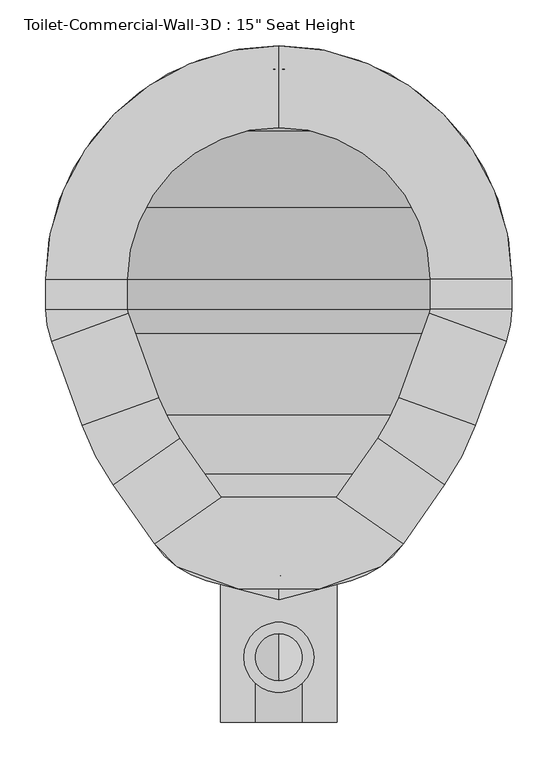
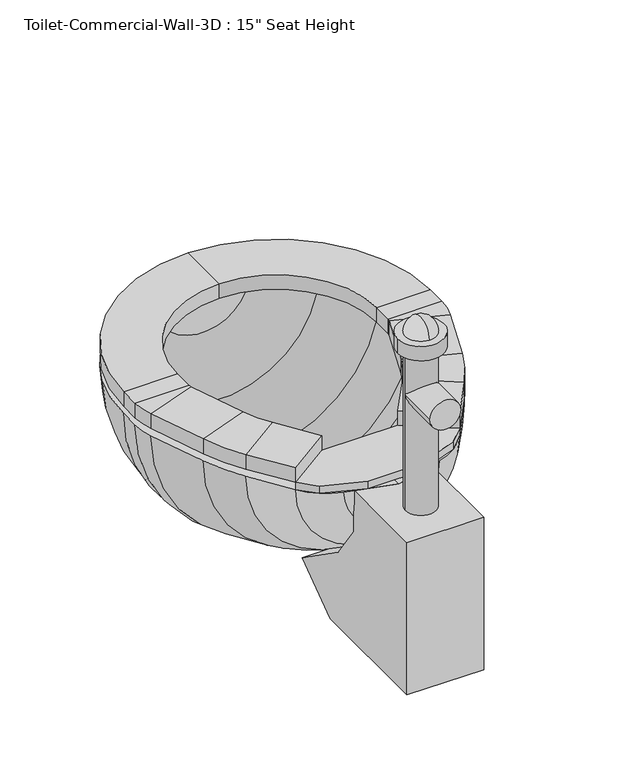
"""IFC4 building model written with IfcOpenShell, lengths in millimetres: flow terminal geometry."""

from ifc_helpers import new_model, si_unit, point, frame, frame_2d, origin, place, context, project, spatial, polyline, circle_curve, ellipse_curve, trimmed, segment, composite_curve, outline, extrude, source, transform, mapped, element, save
from ifc_brep_helpers import plane_surface, cylinder_surface, revolved_surface, advanced_brep


def flow_terminal_6d55091a(model_context):
    return source(origin(), model_context, "Body", "SolidModel", [
        extrude(outline(polyline([(467.7541169, 321.2347495), (540.5767337, 270.2438043), (515.6262519, 245.2933226), (449.563909, 221.2485961), (360.2423986, 221.2485961), (294.1800557, 245.2933226), (269.229574, 270.2438043), (342.0521907, 321.2347495), (467.7541169, 321.2347495)])), frame((0.0, 0.0, 342.9), z_axis=(0.0, 0.0, 1.0), x_axis=(1.0, 0.0, 0.0)), (0.0, 0.0, 1.0), 12.7),
        advanced_brep(
        [(467.7541169, 321.2347495, 355.6), (540.5767337, 270.2438043, 355.6), (540.5767337, 270.2438043, 381.0), (467.7541169, 321.2347495, 381.0), (512.8583992, 385.6503403, 355.6), (585.6810159, 334.6593951, 355.6), (585.6810159, 334.6593951, 381.0), (512.8583992, 385.6503403, 381.0), (619.360053, 399.3562234, 355.6), (535.821379, 429.7618141, 355.6), (619.360053, 399.3562234, 381.0), (535.821379, 429.7618141, 381.0), (569.2372501, 521.5711654, 355.6), (652.7759241, 491.1655747, 355.6), (652.7759241, 491.1655747, 381.0), (569.2372501, 521.5711654, 381.0), (658.9031538, 525.9148212, 355.6), (570.0031538, 525.9148212, 355.6), (658.9031538, 525.9148212, 381.0), (570.0031538, 525.9148212, 381.0), (570.0031538, 558.8, 355.6), (658.9031538, 558.8, 355.6), (658.9031538, 558.8, 381.0), (570.0031538, 558.8, 381.0), (404.9031538, 812.8, 355.6), (404.9031538, 723.9, 355.6), (404.9031538, 812.8, 381.0), (404.9031538, 723.9, 381.0), (150.9031538, 558.8, 355.6), (239.8031538, 558.8, 355.6), (150.9031538, 558.8, 381.0), (239.8031538, 558.8, 381.0), (239.8031538, 525.9148212, 355.6), (150.9031538, 525.9148212, 355.6), (150.9031538, 525.9148212, 381.0), (239.8031538, 525.9148212, 381.0), (157.0303835, 491.1655747, 355.6), (240.5690575, 521.5711654, 355.6), (157.0303835, 491.1655747, 381.0), (240.5690575, 521.5711654, 381.0), (273.9849286, 429.7618141, 355.6), (190.4462546, 399.3562234, 355.6), (190.4462546, 399.3562234, 381.0), (273.9849286, 429.7618141, 381.0), (224.1252917, 334.6593951, 355.6), (296.9479084, 385.6503403, 355.6), (224.1252917, 334.6593951, 381.0), (296.9479084, 385.6503403, 381.0), (342.0521907, 321.2347495, 355.6), (342.0521907, 321.2347495, 381.0), (269.229574, 270.2438043, 381.0), (269.229574, 270.2438043, 355.6)],
        [
            (0, 1),
            (1, 2),
            (2, 3),
            (3, 0),
            (0, 4),
            (4, 5),
            (5, 1),
            (5, 6),
            (6, 2),
            (6, 7),
            (7, 3),
            (7, 4),
            (8, 5, circle_curve(frame((356.8099347, 494.9166514, 355.6), z_axis=(0.0, 0.0, -1.0), x_axis=(0.81915204428899, -0.5735764363510486, 0.0)), 279.4)),
            (4, 9, circle_curve(frame((356.8099347, 494.9166514, 355.6), z_axis=(0.0, 0.0, 1.0), x_axis=(0.81915204428899, -0.5735764363510486, 0.0)), 190.5)),
            (9, 8),
            (10, 6, circle_curve(frame((356.8099347, 494.9166514, 381.0), z_axis=(0.0, 0.0, -1.0), x_axis=(0.81915204428899, -0.5735764363510486, 0.0)), 279.4)),
            (8, 10),
            (11, 7, circle_curve(frame((356.8099347, 494.9166514, 381.0), z_axis=(0.0, 0.0, -1.0), x_axis=(0.81915204428899, -0.5735764363510486, 0.0)), 190.5)),
            (10, 11),
            (11, 9),
            (9, 12),
            (12, 13),
            (13, 8),
            (13, 14),
            (14, 10),
            (14, 15),
            (15, 11),
            (15, 12),
            (16, 13, circle_curve(frame((557.3031538, 525.9148212, 355.6), z_axis=(0.0, 0.0, -1.0), x_axis=(0.939692620785906, -0.34202014332567526, 0.0)), 101.6)),
            (12, 17, circle_curve(frame((557.3031538, 525.9148212, 355.6), z_axis=(0.0, 0.0, 1.0), x_axis=(0.939692620785906, -0.34202014332567526, 0.0)), 12.7)),
            (17, 16),
            (18, 14, circle_curve(frame((557.3031538, 525.9148212, 381.0), z_axis=(0.0, 0.0, -1.0), x_axis=(0.939692620785906, -0.34202014332567526, 0.0)), 101.6)),
            (16, 18),
            (19, 15, circle_curve(frame((557.3031538, 525.9148212, 381.0), z_axis=(0.0, 0.0, -1.0), x_axis=(0.939692620785906, -0.34202014332567526, 0.0)), 12.7)),
            (18, 19),
            (19, 17),
            (17, 20),
            (20, 21),
            (21, 16),
            (21, 22),
            (22, 18),
            (22, 23),
            (23, 19),
            (23, 20),
            (24, 21, circle_curve(frame((404.9031538, 558.8, 355.6), z_axis=(0.0, 0.0, -1.0), x_axis=(1.0, 0.0, 0.0)), 254.0)),
            (20, 25, circle_curve(frame((404.9031538, 558.8, 355.6), z_axis=(0.0, 0.0, 1.0), x_axis=(1.0, 0.0, 0.0)), 165.1)),
            (25, 24),
            (26, 22, circle_curve(frame((404.9031538, 558.8, 381.0), z_axis=(0.0, 0.0, -1.0), x_axis=(1.0, 0.0, 0.0)), 254.0)),
            (24, 26),
            (27, 23, circle_curve(frame((404.9031538, 558.8, 381.0), z_axis=(0.0, 0.0, -1.0), x_axis=(1.0, 0.0, 0.0)), 165.1)),
            (26, 27),
            (27, 25),
            (28, 24, circle_curve(frame((404.9031538, 558.8, 355.6), z_axis=(0.0, 0.0, -1.0), x_axis=(0.0, 1.0, 0.0)), 254.0)),
            (25, 29, circle_curve(frame((404.9031538, 558.8, 355.6), z_axis=(0.0, 0.0, 1.0), x_axis=(0.0, 1.0, 0.0)), 165.1)),
            (29, 28),
            (30, 26, circle_curve(frame((404.9031538, 558.8, 381.0), z_axis=(0.0, 0.0, -1.0), x_axis=(0.0, 1.0, 0.0)), 254.0)),
            (28, 30),
            (31, 27, circle_curve(frame((404.9031538, 558.8, 381.0), z_axis=(0.0, 0.0, -1.0), x_axis=(0.0, 1.0, 0.0)), 165.1)),
            (30, 31),
            (31, 29),
            (29, 32),
            (32, 33),
            (33, 28),
            (33, 34),
            (34, 30),
            (34, 35),
            (35, 31),
            (35, 32),
            (36, 33, circle_curve(frame((252.5031538, 525.9148212, 355.6), z_axis=(0.0, 0.0, -1.0), x_axis=(-1.0, 0.0, 0.0)), 101.6)),
            (32, 37, circle_curve(frame((252.5031538, 525.9148212, 355.6), z_axis=(0.0, 0.0, 1.0), x_axis=(-1.0, 0.0, 0.0)), 12.7)),
            (37, 36),
            (38, 34, circle_curve(frame((252.5031538, 525.9148212, 381.0), z_axis=(0.0, 0.0, -1.0), x_axis=(-1.0, 0.0, 0.0)), 101.6)),
            (36, 38),
            (39, 35, circle_curve(frame((252.5031538, 525.9148212, 381.0), z_axis=(0.0, 0.0, -1.0), x_axis=(-1.0, 0.0, 0.0)), 12.7)),
            (38, 39),
            (39, 37),
            (37, 40),
            (40, 41),
            (41, 36),
            (41, 42),
            (42, 38),
            (42, 43),
            (43, 39),
            (43, 40),
            (44, 41, circle_curve(frame((452.9963729, 494.9166514, 355.6), z_axis=(0.0, 0.0, -1.0), x_axis=(-0.9396926207859088, -0.34202014332566766, 0.0)), 279.4)),
            (40, 45, circle_curve(frame((452.9963729, 494.9166514, 355.6), z_axis=(0.0, 0.0, 1.0), x_axis=(-0.9396926207859088, -0.34202014332566766, 0.0)), 190.5)),
            (45, 44),
            (46, 42, circle_curve(frame((452.9963729, 494.9166514, 381.0), z_axis=(0.0, 0.0, -1.0), x_axis=(-0.9396926207859088, -0.34202014332566766, 0.0)), 279.4)),
            (44, 46),
            (47, 43, circle_curve(frame((452.9963729, 494.9166514, 381.0), z_axis=(0.0, 0.0, -1.0), x_axis=(-0.9396926207859088, -0.34202014332566766, 0.0)), 190.5)),
            (46, 47),
            (47, 45),
            (48, 49),
            (49, 50),
            (50, 51),
            (51, 48),
            (45, 48),
            (51, 44),
            (50, 46),
            (49, 47),
        ],
        [
            plane_surface(frame((540.5767337, 270.2438043, 439.6203184), z_axis=(-0.5735764363510434, -0.8191520442889938, 0.0), x_axis=(0.8191520442889938, -0.5735764363510434, 0.0))),
            plane_surface(frame((467.7541169, 321.2347495, 355.6), z_axis=(0.0, 0.0, -1.0), x_axis=(0.573576436351044, 0.8191520442889932, 0.0))),
            plane_surface(frame((540.5767337, 270.2438043, 355.6), z_axis=(0.8191520442889938, -0.5735764363510433, 0.0), x_axis=(0.5735764363510433, 0.8191520442889938, 0.0))),
            plane_surface(frame((540.5767337, 270.2438043, 381.0), z_axis=(0.0, 0.0, 1.0), x_axis=(0.5735764363510433, 0.8191520442889938, 0.0))),
            plane_surface(frame((467.7541169, 321.2347495, 381.0), z_axis=(-0.8191520442889932, 0.573576436351044, 0.0), x_axis=(0.573576436351044, 0.8191520442889932, 0.0))),
            plane_surface(frame((356.8099347, 494.9166514, 355.6), z_axis=(0.0, 0.0, -1.0), x_axis=(0.81915204428899, -0.5735764363510486, 0.0))),
            cylinder_surface(frame((356.8099347, 494.9166514, 342.9), z_axis=(0.0, 0.0, 1.0), x_axis=(0.81915204428899, -0.5735764363510486, 0.0)), 279.4),
            plane_surface(frame((356.8099347, 494.9166514, 381.0), z_axis=(0.0, 0.0, 1.0), x_axis=(0.81915204428899, -0.5735764363510486, 0.0))),
            revolved_surface(polyline([(512.8583991370526, 385.65034027512525, 381.0), (512.8583991370526, 385.65034027512525, 355.6)]), (356.8099347, 494.9166514, 342.9), (0.0, 0.0, 1.0)),
            plane_surface(frame((535.821379, 429.7618141, 355.6), z_axis=(0.0, 0.0, -1.0000000000000002), x_axis=(0.3420201433256694, 0.9396926207859082, 0.0))),
            plane_surface(frame((619.360053, 399.3562234, 355.6), z_axis=(0.9396926207859075, -0.34202014332567104, 0.0), x_axis=(0.34202014332567104, 0.9396926207859075, 0.0))),
            plane_surface(frame((619.360053, 399.3562234, 381.0), z_axis=(0.0, 0.0, 1.0), x_axis=(0.3420201433256696, 0.9396926207859081, 0.0))),
            plane_surface(frame((535.821379, 429.7618141, 381.0), z_axis=(-0.939692620785908, 0.34202014332567, 0.0), x_axis=(0.34202014332567, 0.939692620785908, 0.0))),
            plane_surface(frame((557.3031538, 525.9148212, 355.6), z_axis=(0.0, 0.0, -1.0), x_axis=(0.939692620785906, -0.34202014332567526, 0.0))),
            cylinder_surface(frame((557.3031538, 525.9148212, 342.9), z_axis=(0.0, 0.0, 1.0), x_axis=(0.939692620785906, -0.34202014332567526, 0.0)), 101.6),
            plane_surface(frame((557.3031538, 525.9148212, 381.0), z_axis=(0.0, 0.0, 1.0), x_axis=(0.939692620785906, -0.34202014332567526, 0.0))),
            revolved_surface(polyline([(569.237250083981, 521.5711653797639, 381.0), (569.237250083981, 521.5711653797639, 355.6)]), (557.3031538, 525.9148212, 342.9), (0.0, 0.0, 1.0)),
            plane_surface(frame((570.0031538, 525.9148212, 355.6), z_axis=(0.0, 0.0, -1.0), x_axis=(0.0, 1.0, 0.0))),
            plane_surface(frame((658.9031538, 525.9148212, 355.6), z_axis=(1.0, 0.0, 0.0), x_axis=(0.0, 1.0, 0.0))),
            plane_surface(frame((658.9031538, 525.9148212, 381.0), z_axis=(0.0, 0.0, 1.0), x_axis=(0.0, 1.0, 0.0))),
            plane_surface(frame((570.0031538, 525.9148212, 381.0), z_axis=(-1.0, 0.0, 0.0), x_axis=(0.0, 1.0, 0.0))),
            plane_surface(frame((404.9031538, 558.8, 355.6), z_axis=(0.0, 0.0, -1.0), x_axis=(1.0, 0.0, 0.0))),
            cylinder_surface(frame((404.9031538, 558.8, 342.9), z_axis=(0.0, 0.0, 1.0), x_axis=(1.0, 0.0, 0.0)), 254.0),
            plane_surface(frame((404.9031538, 558.8, 381.0), z_axis=(0.0, 0.0, 1.0), x_axis=(1.0, 0.0, 0.0))),
            revolved_surface(polyline([(570.0031538, 558.8, 381.0), (570.0031538, 558.8, 355.6)]), (404.9031538, 558.8, 342.9), (0.0, 0.0, 1.0)),
            plane_surface(frame((404.9031538, 558.8, 355.6), z_axis=(0.0, 0.0, -1.0), x_axis=(0.0, 1.0, 0.0))),
            cylinder_surface(frame((404.9031538, 558.8, 342.9), z_axis=(0.0, 0.0, 1.0), x_axis=(0.0, 1.0, 0.0)), 254.0),
            plane_surface(frame((404.9031538, 558.8, 381.0), z_axis=(0.0, 0.0, 1.0), x_axis=(0.0, 1.0, 0.0))),
            revolved_surface(polyline([(404.9031538, 723.9, 381.0), (404.9031538, 723.9, 355.6)]), (404.9031538, 558.8, 342.9), (0.0, 0.0, 1.0)),
            plane_surface(frame((239.8031538, 558.8, 355.6), z_axis=(0.0, 0.0, -1.0), x_axis=(0.0, -1.0, 0.0))),
            plane_surface(frame((150.9031538, 558.8, 355.6), z_axis=(-1.0, 0.0, 0.0), x_axis=(0.0, -1.0, 0.0))),
            plane_surface(frame((150.9031538, 558.8, 381.0), z_axis=(0.0, 0.0, 1.0), x_axis=(0.0, -1.0, 0.0))),
            plane_surface(frame((239.8031538, 558.8, 381.0), z_axis=(1.0, 0.0, 0.0), x_axis=(0.0, -1.0, 0.0))),
            plane_surface(frame((252.5031538, 525.9148212, 355.6), z_axis=(0.0, 0.0, -1.0), x_axis=(-1.0, 0.0, 0.0))),
            cylinder_surface(frame((252.5031538, 525.9148212, 342.9), z_axis=(0.0, 0.0, 1.0), x_axis=(-1.0, 0.0, 0.0)), 101.6),
            plane_surface(frame((252.5031538, 525.9148212, 381.0), z_axis=(0.0, 0.0, 1.0), x_axis=(-1.0, 0.0, 0.0))),
            revolved_surface(polyline([(239.80315380000002, 525.9148212, 381.0), (239.80315380000002, 525.9148212, 355.6)]), (252.5031538, 525.9148212, 342.9), (0.0, 0.0, 1.0)),
            plane_surface(frame((240.5690575, 521.5711654, 355.6), z_axis=(0.0, 0.0, -1.0), x_axis=(0.3420201433256672, -0.939692620785909, 0.0))),
            plane_surface(frame((157.0303835, 491.1655747, 355.6), z_axis=(-0.9396926207859091, -0.3420201433256668, 0.0), x_axis=(0.3420201433256668, -0.9396926207859091, 0.0))),
            plane_surface(frame((157.0303835, 491.1655747, 381.0), z_axis=(0.0, 0.0, 1.0), x_axis=(0.3420201433256671, -0.939692620785909, 0.0))),
            plane_surface(frame((240.5690575, 521.5711654, 381.0), z_axis=(0.9396926207859091, 0.342020143325667, 0.0), x_axis=(0.342020143325667, -0.9396926207859091, 0.0))),
            plane_surface(frame((452.9963729, 494.9166514, 355.6), z_axis=(0.0, 0.0, -1.0), x_axis=(-0.9396926207859088, -0.34202014332566766, 0.0))),
            cylinder_surface(frame((452.9963729, 494.9166514, 342.9), z_axis=(0.0, 0.0, 1.0), x_axis=(-0.9396926207859088, -0.34202014332566766, 0.0)), 279.4),
            plane_surface(frame((452.9963729, 494.9166514, 381.0), z_axis=(0.0, 0.0, 1.0), x_axis=(-0.9396926207859088, -0.34202014332566766, 0.0))),
            revolved_surface(polyline([(273.98492864028435, 429.7618140964603, 381.0), (273.98492864028435, 429.7618140964603, 355.6)]), (452.9963729, 494.9166514, 342.9), (0.0, 0.0, 1.0)),
            plane_surface(frame((269.229574, 270.2438043, 246.1796816), z_axis=(0.5735764363510462, -0.8191520442889919, 0.0), x_axis=(0.8191520442889919, 0.5735764363510462, 0.0))),
            plane_surface(frame((296.9479084, 385.6503403, 355.6), z_axis=(0.0, 0.0, -1.0), x_axis=(0.5735764363510465, -0.8191520442889916, 0.0))),
            plane_surface(frame((224.1252917, 334.6593951, 355.6), z_axis=(-0.8191520442889917, -0.5735764363510464, 0.0), x_axis=(0.5735764363510464, -0.8191520442889917, 0.0))),
            plane_surface(frame((224.1252917, 334.6593951, 381.0), z_axis=(0.0, 0.0, 1.0000000000000002), x_axis=(0.5735764363510462, -0.8191520442889919, 0.0))),
            plane_surface(frame((296.9479084, 385.6503403, 381.0), z_axis=(0.8191520442889916, 0.5735764363510465, 0.0), x_axis=(0.5735764363510465, -0.8191520442889916, 0.0))),
        ],
        [
            (0, [[1, 2, 3, 4]]),
            (1, [[-1, 5, 6, 7]]),
            (2, [[-2, -7, 8, 9]]),
            (3, [[-3, -9, 10, 11]]),
            (4, [[-4, -11, 12, -5]]),
            (5, [[13, -6, 14, 15]]),
            (6, [[16, -8, -13, 17]]),
            (7, [[18, -10, -16, 19]]),
            (8, [[-14, -12, -18, 20]]),
            (9, [[-15, 21, 22, 23]]),
            (10, [[-17, -23, 24, 25]]),
            (11, [[-19, -25, 26, 27]]),
            (12, [[-20, -27, 28, -21]]),
            (13, [[29, -22, 30, 31]]),
            (14, [[32, -24, -29, 33]]),
            (15, [[34, -26, -32, 35]]),
            (16, [[-30, -28, -34, 36]]),
            (17, [[-31, 37, 38, 39]]),
            (18, [[-33, -39, 40, 41]]),
            (19, [[-35, -41, 42, 43]]),
            (20, [[-36, -43, 44, -37]]),
            (21, [[45, -38, 46, 47]]),
            (22, [[48, -40, -45, 49]]),
            (23, [[50, -42, -48, 51]]),
            (24, [[-46, -44, -50, 52]]),
            (25, [[53, -47, 54, 55]]),
            (26, [[56, -49, -53, 57]]),
            (27, [[58, -51, -56, 59]]),
            (28, [[-54, -52, -58, 60]]),
            (29, [[-55, 61, 62, 63]]),
            (30, [[-57, -63, 64, 65]]),
            (31, [[-59, -65, 66, 67]]),
            (32, [[-60, -67, 68, -61]]),
            (33, [[69, -62, 70, 71]]),
            (34, [[72, -64, -69, 73]]),
            (35, [[74, -66, -72, 75]]),
            (36, [[-70, -68, -74, 76]]),
            (37, [[-71, 77, 78, 79]]),
            (38, [[-73, -79, 80, 81]]),
            (39, [[-75, -81, 82, 83]]),
            (40, [[-76, -83, 84, -77]]),
            (41, [[85, -78, 86, 87]]),
            (42, [[88, -80, -85, 89]]),
            (43, [[90, -82, -88, 91]]),
            (44, [[-86, -84, -90, 92]]),
            (45, [[93, 94, 95, 96]]),
            (46, [[-87, 97, -96, 98]]),
            (47, [[-89, -98, -95, 99]]),
            (48, [[-91, -99, -94, 100]]),
            (49, [[-92, -100, -93, -97]]),
        ],
    ),
        advanced_brep(
        [(491.7762702, 797.4819257, 342.9), (404.9031538, 812.8, 342.9), (404.9031538, 787.4, 342.9), (483.0889586, 773.6137331, 342.9), (566.547764, 720.4446102, 342.9), (619.7168869, 636.9858048, 342.9), (633.5031538, 558.8, 342.9), (633.5031538, 525.9148212, 342.9), (628.9077315, 499.8528863, 342.9), (596.6355667, 411.1858422, 342.9), (562.9565296, 346.4890139, 342.9), (525.0728964, 292.3855786, 342.9), (468.1430637, 252.5228806, 342.9), (404.9031538, 235.5777978, 342.9), (404.9031538, 209.2817829, 342.9), (483.6469009, 230.3811063, 342.9), (540.5767337, 270.2438043, 342.9), (585.6810159, 334.6593951, 342.9), (619.360053, 399.3562234, 342.9), (652.7759241, 491.1655747, 342.9), (658.9031538, 525.9148212, 342.9), (658.9031538, 558.8, 342.9), (643.5850795, 645.6731164, 342.9), (584.5082762, 738.4051224, 342.9), (318.0300374, 797.4819257, 342.9), (225.2980314, 738.4051224, 342.9), (166.2212281, 645.6731164, 342.9), (150.9031538, 558.8, 342.9), (150.9031538, 525.9148212, 342.9), (157.0303835, 491.1655747, 342.9), (190.4462546, 399.3562234, 342.9), (224.1252917, 334.6593951, 342.9), (269.229574, 270.2438043, 342.9), (326.1594067, 230.3811063, 342.9), (341.663244, 252.5228806, 342.9), (284.7334112, 292.3855786, 342.9), (246.849778, 346.4890139, 342.9), (213.1707409, 411.1858422, 342.9), (180.8985761, 499.8528863, 342.9), (176.3031538, 525.9148212, 342.9), (176.3031538, 558.8, 342.9), (190.0894207, 636.9858048, 342.9), (243.2585436, 720.4446102, 342.9), (326.7173491, 773.6137331, 342.9)],
        [
            (0, 1, circle_curve(frame((404.9031538, 558.8, 342.9), z_axis=(0.0, 0.0, 1.0), x_axis=(1.0, 0.0, 0.0)), 254.0)),
            (1, 2),
            (2, 3, circle_curve(frame((404.9031538, 558.8, 342.9), z_axis=(0.0, 0.0, -1.0), x_axis=(1.0, 0.0, 0.0)), 228.6)),
            (3, 4, circle_curve(frame((404.9031538, 558.8, 342.9), z_axis=(0.0, 0.0, -1.0), x_axis=(1.0, 0.0, 0.0)), 228.6)),
            (4, 5, circle_curve(frame((404.9031538, 558.8, 342.9), z_axis=(0.0, 0.0, -1.0), x_axis=(1.0, 0.0, 0.0)), 228.6)),
            (5, 6, circle_curve(frame((404.9031538, 558.8, 342.9), z_axis=(0.0, 0.0, -1.0), x_axis=(1.0, 0.0, 0.0)), 228.6)),
            (6, 7),
            (7, 8, circle_curve(frame((557.3031538, 525.9148212, 342.9), z_axis=(0.0, 0.0, -1.0), x_axis=(1.0, 0.0, 0.0)), 76.2)),
            (8, 9),
            (9, 10, circle_curve(frame((334.0854485, 506.7462703, 342.9), z_axis=(0.0, 0.0, -1.0), x_axis=(1.0, 0.0, 0.0)), 279.4)),
            (10, 11),
            (11, 12, circle_curve(frame((441.8470487, 350.6609446, 342.9), z_axis=(0.0, 0.0, -1.0), x_axis=(1.0, 0.0, 0.0)), 101.6)),
            (12, 13),
            (13, 14),
            (14, 15),
            (15, 16, circle_curve(frame((457.350886, 328.5191703, 342.9), z_axis=(0.0, 0.0, 1.0), x_axis=(1.0, 0.0, 0.0)), 101.6)),
            (16, 17),
            (17, 18, circle_curve(frame((356.8099347, 494.9166514, 342.9), z_axis=(0.0, 0.0, 1.0), x_axis=(1.0, 0.0, 0.0)), 279.4)),
            (18, 19),
            (19, 20, circle_curve(frame((557.3031538, 525.9148212, 342.9), z_axis=(0.0, 0.0, 1.0), x_axis=(1.0, 0.0, 0.0)), 101.6)),
            (20, 21),
            (21, 22, circle_curve(frame((404.9031538, 558.8, 342.9), z_axis=(0.0, 0.0, 1.0), x_axis=(1.0, 0.0, 0.0)), 254.0)),
            (22, 23, circle_curve(frame((404.9031538, 558.8, 342.9), z_axis=(0.0, 0.0, 1.0), x_axis=(1.0, 0.0, 0.0)), 254.0)),
            (23, 0, circle_curve(frame((404.9031538, 558.8, 342.9), z_axis=(0.0, 0.0, 1.0), x_axis=(1.0, 0.0, 0.0)), 254.0)),
            (24, 25, circle_curve(frame((404.9031538, 558.8, 342.9), z_axis=(0.0, 0.0, 1.0), x_axis=(-1.0, 0.0, 0.0)), 254.0)),
            (25, 26, circle_curve(frame((404.9031538, 558.8, 342.9), z_axis=(0.0, 0.0, 1.0), x_axis=(-1.0, 0.0, 0.0)), 254.0)),
            (26, 27, circle_curve(frame((404.9031538, 558.8, 342.9), z_axis=(0.0, 0.0, 1.0), x_axis=(-1.0, 0.0, 0.0)), 254.0)),
            (27, 28),
            (28, 29, circle_curve(frame((252.5031538, 525.9148212, 342.9), z_axis=(0.0, 0.0, 1.0), x_axis=(-1.0, 0.0, 0.0)), 101.6)),
            (29, 30),
            (30, 31, circle_curve(frame((452.9963729, 494.9166514, 342.9), z_axis=(0.0, 0.0, 1.0), x_axis=(-1.0, 0.0, 0.0)), 279.4)),
            (31, 32),
            (32, 33, circle_curve(frame((352.4554217, 328.5191703, 342.9), z_axis=(0.0, 0.0, 1.0), x_axis=(-1.0, 0.0, 0.0)), 101.6)),
            (33, 14),
            (13, 34),
            (34, 35, circle_curve(frame((367.9592589, 350.6609446, 342.9), z_axis=(0.0, 0.0, -1.0), x_axis=(-1.0, 0.0, 0.0)), 101.6)),
            (35, 36),
            (36, 37, circle_curve(frame((475.7208592, 506.7462703, 342.9), z_axis=(0.0, 0.0, -1.0), x_axis=(-1.0, 0.0, 0.0)), 279.4)),
            (37, 38),
            (38, 39, circle_curve(frame((252.5031538, 525.9148212, 342.9), z_axis=(0.0, 0.0, -1.0), x_axis=(-1.0, 0.0, 0.0)), 76.2)),
            (39, 40),
            (40, 41, circle_curve(frame((404.9031538, 558.8, 342.9), z_axis=(0.0, 0.0, -1.0), x_axis=(-1.0, 0.0, 0.0)), 228.6)),
            (41, 42, circle_curve(frame((404.9031538, 558.8, 342.9), z_axis=(0.0, 0.0, -1.0), x_axis=(-1.0, 0.0, 0.0)), 228.6)),
            (42, 43, circle_curve(frame((404.9031538, 558.8, 342.9), z_axis=(0.0, 0.0, -1.0), x_axis=(-1.0, 0.0, 0.0)), 228.6)),
            (43, 2, circle_curve(frame((404.9031538, 558.8, 342.9), z_axis=(0.0, 0.0, -1.0), x_axis=(-1.0, 0.0, 0.0)), 228.6)),
            (1, 24, circle_curve(frame((404.9031538, 558.8, 342.9), z_axis=(0.0, 0.0, 1.0), x_axis=(-1.0, 0.0, 0.0)), 254.0)),
            (0, 24, circle_curve(frame((404.9031538, 797.4819257, 342.9), z_axis=(0.0, 1.0, 0.0), x_axis=(1.0, 0.0, 0.0)), 86.8731164)),
            (43, 3, circle_curve(frame((404.9031538, 773.6137331, 342.9), z_axis=(0.0, -1.0, 0.0), x_axis=(1.0, 0.0, 0.0)), 78.1858048)),
            (42, 4, circle_curve(frame((404.9031538, 720.4446102, 342.9), z_axis=(0.0, -1.0, 0.0), x_axis=(1.0, 0.0, 0.0)), 161.6446102)),
            (41, 5, circle_curve(frame((404.9031538, 636.9858048, 342.9), z_axis=(0.0, -1.0, 0.0), x_axis=(1.0, 0.0, 0.0)), 214.8137331)),
            (40, 6, circle_curve(frame((404.9031538, 558.8, 342.9), z_axis=(0.0, -1.0, 0.0), x_axis=(1.0, 0.0, 0.0)), 228.6)),
            (39, 7, circle_curve(frame((404.9031538, 525.9148212, 342.9), z_axis=(0.0, -1.0, 0.0), x_axis=(1.0, 0.0, 0.0)), 228.6)),
            (38, 8, circle_curve(frame((404.9031538, 499.8528863, 342.9), z_axis=(0.0, -1.0, 0.0), x_axis=(1.0, 0.0, 0.0)), 224.0045777)),
            (37, 9, circle_curve(frame((404.9031538, 411.1858422, 342.9), z_axis=(0.0, -1.0, 0.0), x_axis=(1.0, 0.0, 0.0)), 191.7324129)),
            (36, 10, circle_curve(frame((404.9031538, 346.4890139, 342.9), z_axis=(0.0, -1.0, 0.0), x_axis=(1.0, 0.0, 0.0)), 158.0533758)),
            (35, 11, circle_curve(frame((404.9031538, 292.3855786, 342.9), z_axis=(0.0, -1.0, 0.0), x_axis=(1.0, 0.0, 0.0)), 120.1697426)),
            (34, 12, circle_curve(frame((404.9031538, 252.5228806, 342.9), z_axis=(0.0, -1.0, 0.0), x_axis=(1.0, 0.0, 0.0)), 63.2399099)),
            (33, 15, circle_curve(frame((404.9031538, 230.3811063, 342.9), z_axis=(0.0, -1.0, 0.0), x_axis=(1.0, 0.0, 0.0)), 78.7437471)),
            (32, 16, circle_curve(frame((404.9031538, 270.2438043, 342.9), z_axis=(0.0, -1.0, 0.0), x_axis=(1.0, 0.0, 0.0)), 135.6735798)),
            (31, 17, circle_curve(frame((404.9031538, 334.6593951, 342.9), z_axis=(0.0, -1.0, 0.0), x_axis=(1.0, 0.0, 0.0)), 180.7778621)),
            (30, 18, circle_curve(frame((404.9031538, 399.3562234, 342.9), z_axis=(0.0, -1.0, 0.0), x_axis=(1.0, 0.0, 0.0)), 214.4568992)),
            (29, 19, circle_curve(frame((404.9031538, 491.1655747, 342.9), z_axis=(0.0, -1.0, 0.0), x_axis=(1.0, 0.0, 0.0)), 247.8727703)),
            (28, 20, circle_curve(frame((404.9031538, 525.9148212, 342.9), z_axis=(0.0, -1.0, 0.0), x_axis=(1.0, 0.0, 0.0)), 254.0)),
            (27, 21, circle_curve(frame((404.9031538, 558.8, 342.9), z_axis=(0.0, -1.0, 0.0), x_axis=(1.0, 0.0, 0.0)), 254.0)),
            (26, 22, circle_curve(frame((404.9031538, 645.6731164, 342.9), z_axis=(0.0, -1.0, 0.0), x_axis=(1.0, 0.0, 0.0)), 238.6819257)),
            (25, 23, circle_curve(frame((404.9031538, 738.4051224, 342.9), z_axis=(0.0, -1.0, 0.0), x_axis=(1.0, 0.0, 0.0)), 179.6051224)),
        ],
        [
            plane_surface(frame((404.9031538, 918.0102448, 342.9), z_axis=(0.0, 0.0, 1.0), x_axis=(1.0, 0.0, 0.0))),
            plane_surface(frame((404.9031538, 918.0102448, 342.9), z_axis=(0.0, 0.0, 1.0), x_axis=(-1.0, 0.0, 0.0))),
            revolved_surface(trimmed(ellipse_curve(frame((404.9031538, 558.8, 342.9), z_axis=(0.0, 0.0, 1.0), x_axis=(1.0, 0.0, 0.0)), 254.0, 254.0), [point((491.7762702, 797.4819257, 342.9))], [point((404.9031538, 812.8, 342.9))], True, "CARTESIAN"), (404.9031538, 918.0102448, 342.9), (0.0, 1.0, 0.0)),
            revolved_surface(trimmed(ellipse_curve(frame((404.9031538, 558.8, 342.9), z_axis=(0.0, 0.0, -1.0), x_axis=(1.0, 0.0, 0.0)), 228.6, 228.6), [point((404.9031538, 787.4, 342.9))], [point((483.0889586, 773.6137331, 342.9))], True, "CARTESIAN"), (404.9031538, 918.0102448, 342.9), (0.0, 1.0, 0.0)),
            revolved_surface(trimmed(ellipse_curve(frame((404.9031538, 558.8, 342.9), z_axis=(0.0, 0.0, -1.0), x_axis=(1.0, 0.0, 0.0)), 228.6, 228.6), [point((483.0889586, 773.6137331, 342.9))], [point((566.547764, 720.4446102, 342.9))], True, "CARTESIAN"), (404.9031538, 918.0102448, 342.9), (0.0, 1.0, 0.0)),
            revolved_surface(trimmed(ellipse_curve(frame((404.9031538, 558.8, 342.9), z_axis=(0.0, 0.0, -1.0), x_axis=(1.0, 0.0, 0.0)), 228.6, 228.6), [point((566.547764, 720.4446102, 342.9))], [point((619.7168869, 636.9858048, 342.9))], True, "CARTESIAN"), (404.9031538, 918.0102448, 342.9), (0.0, 1.0, 0.0)),
            revolved_surface(trimmed(ellipse_curve(frame((404.9031538, 558.8, 342.9), z_axis=(0.0, 0.0, -1.0), x_axis=(1.0, 0.0, 0.0)), 228.6, 228.6), [point((619.7168869, 636.9858048, 342.9))], [point((633.5031538, 558.8, 342.9))], True, "CARTESIAN"), (404.9031538, 918.0102448, 342.9), (0.0, 1.0, 0.0)),
            revolved_surface(polyline([(633.5031538, 558.8, 342.9), (633.5031538, 525.9148212, 342.9)]), (404.9031538, 918.0102448, 342.9), (0.0, 1.0, 0.0)),
            revolved_surface(trimmed(ellipse_curve(frame((557.3031538, 525.9148212, 342.9), z_axis=(0.0, 0.0, -1.0), x_axis=(1.0, 0.0, 0.0)), 76.2, 76.2), [point((633.5031538, 525.9148212, 342.9))], [point((628.9077315, 499.8528863, 342.9))], True, "CARTESIAN"), (404.9031538, 918.0102448, 342.9), (0.0, 1.0, 0.0)),
            revolved_surface(polyline([(628.9077315, 499.8528863, 342.9), (596.6355667, 411.1858422, 342.9)]), (404.9031538, 918.0102448, 342.9), (0.0, 1.0, 0.0)),
            revolved_surface(trimmed(ellipse_curve(frame((334.0854485, 506.7462703, 342.9), z_axis=(0.0, 0.0, -1.0), x_axis=(1.0, 0.0, 0.0)), 279.4, 279.4), [point((596.6355667, 411.1858422, 342.9))], [point((562.9565296, 346.4890139, 342.9))], True, "CARTESIAN"), (404.9031538, 918.0102448, 342.9), (0.0, 1.0, 0.0)),
            revolved_surface(polyline([(562.9565296, 346.4890139, 342.9), (525.0728964, 292.3855786, 342.9)]), (404.9031538, 918.0102448, 342.9), (0.0, 1.0, 0.0)),
            revolved_surface(trimmed(ellipse_curve(frame((441.8470487, 350.6609446, 342.9), z_axis=(0.0, 0.0, -1.0), x_axis=(1.0, 0.0, 0.0)), 101.6, 101.6), [point((525.0728964, 292.3855786, 342.9))], [point((468.1430637, 252.5228806, 342.9))], True, "CARTESIAN"), (404.9031538, 918.0102448, 342.9), (0.0, 1.0, 0.0)),
            revolved_surface(polyline([(468.1430637, 252.5228806, 342.9), (404.9031538, 235.5777978, 342.9)]), (404.9031538, 918.0102448, 342.9), (0.0, 1.0, 0.0)),
            revolved_surface(polyline([(404.9031538, 209.2817829, 342.9), (483.6469009, 230.3811063, 342.9)]), (404.9031538, 918.0102448, 342.9), (0.0, 1.0, 0.0)),
            revolved_surface(trimmed(ellipse_curve(frame((457.350886, 328.5191703, 342.9), z_axis=(0.0, 0.0, 1.0), x_axis=(1.0, 0.0, 0.0)), 101.6, 101.6), [point((483.6469009, 230.3811063, 342.9))], [point((540.5767337, 270.2438043, 342.9))], True, "CARTESIAN"), (404.9031538, 918.0102448, 342.9), (0.0, 1.0, 0.0)),
            revolved_surface(polyline([(540.5767337, 270.2438043, 342.9), (585.6810159, 334.6593951, 342.9)]), (404.9031538, 918.0102448, 342.9), (0.0, 1.0, 0.0)),
            revolved_surface(trimmed(ellipse_curve(frame((356.8099347, 494.9166514, 342.9), z_axis=(0.0, 0.0, 1.0), x_axis=(1.0, 0.0, 0.0)), 279.4, 279.4), [point((585.6810159, 334.6593951, 342.9))], [point((619.360053, 399.3562234, 342.9))], True, "CARTESIAN"), (404.9031538, 918.0102448, 342.9), (0.0, 1.0, 0.0)),
            revolved_surface(polyline([(619.360053, 399.3562234, 342.9), (652.7759241, 491.1655747, 342.9)]), (404.9031538, 918.0102448, 342.9), (0.0, 1.0, 0.0)),
            revolved_surface(trimmed(ellipse_curve(frame((557.3031538, 525.9148212, 342.9), z_axis=(0.0, 0.0, 1.0), x_axis=(1.0, 0.0, 0.0)), 101.6, 101.6), [point((652.7759241, 491.1655747, 342.9))], [point((658.9031538, 525.9148212, 342.9))], True, "CARTESIAN"), (404.9031538, 918.0102448, 342.9), (0.0, 1.0, 0.0)),
            cylinder_surface(frame((404.9031538, 918.0102448, 342.9), z_axis=(0.0, 1.0, 0.0), x_axis=(1.0, 0.0, 0.0)), 254.0),
            revolved_surface(trimmed(ellipse_curve(frame((404.9031538, 558.8, 342.9), z_axis=(0.0, 0.0, 1.0), x_axis=(1.0, 0.0, 0.0)), 254.0, 254.0), [point((658.9031538, 558.8, 342.9))], [point((643.5850795, 645.6731164, 342.9))], True, "CARTESIAN"), (404.9031538, 918.0102448, 342.9), (0.0, 1.0, 0.0)),
            revolved_surface(trimmed(ellipse_curve(frame((404.9031538, 558.8, 342.9), z_axis=(0.0, 0.0, 1.0), x_axis=(1.0, 0.0, 0.0)), 254.0, 254.0), [point((643.5850795, 645.6731164, 342.9))], [point((584.5082762, 738.4051224, 342.9))], True, "CARTESIAN"), (404.9031538, 918.0102448, 342.9), (0.0, 1.0, 0.0)),
            revolved_surface(trimmed(ellipse_curve(frame((404.9031538, 558.8, 342.9), z_axis=(0.0, 0.0, 1.0), x_axis=(1.0, 0.0, 0.0)), 254.0, 254.0), [point((584.5082762, 738.4051224, 342.9))], [point((491.7762702, 797.4819257, 342.9))], True, "CARTESIAN"), (404.9031538, 918.0102448, 342.9), (0.0, 1.0, 0.0)),
        ],
        [
            (0, [[1, 2, 3, 4, 5, 6, 7, 8, 9, 10, 11, 12, 13, 14, 15, 16, 17, 18, 19, 20, 21, 22, 23, 24]]),
            (1, [[25, 26, 27, 28, 29, 30, 31, 32, 33, 34, -14, 35, 36, 37, 38, 39, 40, 41, 42, 43, 44, 45, -2, 46]]),
            (2, [[-1, 47, -46]]),
            (3, [[48, -3, -45]]),
            (4, [[49, -4, -48, -44]]),
            (5, [[50, -5, -49, -43]]),
            (6, [[51, -6, -50, -42]]),
            (7, [[52, -7, -51, -41]]),
            (8, [[53, -8, -52, -40]]),
            (9, [[54, -9, -53, -39]]),
            (10, [[55, -10, -54, -38]]),
            (11, [[56, -11, -55, -37]]),
            (12, [[57, -12, -56, -36]]),
            (13, [[-13, -57, -35]]),
            (14, [[58, -15, -34]]),
            (15, [[59, -16, -58, -33]]),
            (16, [[60, -17, -59, -32]]),
            (17, [[61, -18, -60, -31]]),
            (18, [[62, -19, -61, -30]]),
            (19, [[63, -20, -62, -29]]),
            (20, [[64, -21, -63, -28]]),
            (21, [[65, -22, -64, -27]]),
            (22, [[66, -23, -65, -26]]),
            (23, [[-47, -24, -66, -25]]),
        ],
    ),
        advanced_brep(
        [(404.9031538, 121.1176912, 647.7), (404.9031538, 172.3528563, 647.7), (404.9031538, 146.7352737, 673.3175826), (404.9031538, 146.7352737, 647.7)],
        [
            (0, 1, circle_curve(frame((404.9031538, 146.7352737, 647.7), z_axis=(0.0, 0.0, 1.0), x_axis=(0.0, 1.0, 0.0)), 25.6175826)),
            (1, 2, circle_curve(frame((404.9031538, 146.7352737, 647.7), z_axis=(1.0, 0.0, 0.0), x_axis=(0.0, -1.0, 0.0)), 25.6175826)),
            (2, 0, circle_curve(frame((404.9031538, 146.7352737, 647.7), z_axis=(1.0, 0.0, 0.0), x_axis=(0.0, 1.0, 0.0)), 25.6175826)),
            (1, 0, circle_curve(frame((404.9031538, 146.7352737, 647.7), z_axis=(0.0, 0.0, 1.0), x_axis=(0.0, 1.0, 0.0)), 25.6175826)),
            (3, 1),
            (0, 3),
        ],
        [
            revolved_surface(trimmed(ellipse_curve(frame((404.9031538, 146.7352737, 647.7), z_axis=(-1.0, 0.0, 0.0), x_axis=(0.0, -1.0, 0.0)), 25.6175826, 25.6175826), [point((404.9031538, 146.7352737, 673.3175826))], [point((404.9031538, 172.3528563, 647.7))], True, "CARTESIAN"), (404.9031538, 146.7352737, 712.3277273), (0.0, 0.0, -1.0)),
            plane_surface(frame((404.9031538, 146.7352737, 647.7), z_axis=(0.0, 0.0, -1.0), x_axis=(0.0, 1.0, 0.0))),
        ],
        [
            (0, [[1, 2, 3]]),
            (0, [[4, -3, -2]]),
            (1, [[5, -1, 6]]),
            (1, [[-6, -4, -5]]),
        ],
    ),
        extrude(outline(composite_curve([segment(trimmed(circle_curve(frame_2d((404.9031538, 146.7352737)), 38.1), [point((366.8031538, 146.7352737))], [point((443.0031538, 146.7352737))], False, "CARTESIAN"), True, "CONTINUOUS"), segment(trimmed(circle_curve(frame_2d((404.9031538, 146.7352737)), 38.1), [point((443.0031538, 146.7352737))], [point((366.8031538, 146.7352737))], False, "CARTESIAN"), True, "CONTINUOUS")], self_intersect=False)), frame((0.0, 0.0, 622.3), z_axis=(0.0, 0.0, 1.0), x_axis=(1.0, 0.0, 0.0)), (0.0, 0.0, 1.0), 25.4),
        extrude(outline(composite_curve([segment(trimmed(circle_curve(frame_2d((544.2113641, 404.9031538)), 25.4), [point((544.2113641, 379.5031538))], [point((544.2113641, 430.3031538))], False, "CARTESIAN"), True, "CONTINUOUS"), segment(trimmed(circle_curve(frame_2d((544.2113641, 404.9031538)), 25.4), [point((544.2113641, 430.3031538))], [point((544.2113641, 379.5031538))], False, "CARTESIAN"), True, "CONTINUOUS")], self_intersect=False)), frame((0.0, 76.2, 0.0), z_axis=(0.0, 1.0, 0.0), x_axis=(0.0, 0.0, 1.0)), (0.0, 0.0, 1.0), 70.64375),
        extrude(outline(composite_curve([segment(trimmed(circle_curve(frame_2d((404.9031538, 146.7352737)), 25.4), [point((379.5031538, 146.7352737))], [point((430.3031538, 146.7352737))], False, "CARTESIAN"), True, "CONTINUOUS"), segment(trimmed(circle_curve(frame_2d((404.9031538, 146.7352737)), 25.4), [point((430.3031538, 146.7352737))], [point((379.5031538, 146.7352737))], False, "CARTESIAN"), True, "CONTINUOUS")], self_intersect=False)), frame((0.0, 0.0, 342.9), z_axis=(0.0, 0.0, 1.0), x_axis=(1.0, 0.0, 0.0)), (0.0, 0.0, 1.0), 279.4),
        extrude(outline(polyline([(229.0037941, 342.9), (229.0037941, 269.296452), (272.7103185, 206.8770663), (376.7426282, 134.0328588), (296.2454017, 76.2), (76.2, 76.2), (76.2, 342.9), (229.0037941, 342.9)])), frame((341.4031538, 0.0, 0.0), z_axis=(1.0, 0.0, 0.0), x_axis=(0.0, 1.0, 0.0)), (0.0, 0.0, 1.0), 127.0),
    ])


if __name__ == "__main__":
    model = new_model("IFC4")
    model_context = context("Model", 3, world=origin())
    ifc_project = project(units=[si_unit("LENGTHUNIT", "METRE", prefix="MILLI")], contexts=[model_context])
    site = spatial("IfcSite", under=ifc_project)
    building = spatial("IfcBuilding", under=site)
    placement = place(None, origin())
    flow_terminal_shape = flow_terminal_6d55091a(model_context)
    element("IfcFlowTerminal", 1, ObjectType="Toilet-Commercial-Wall-3D : 15\" Seat Height", at=placement, inside=building, context=model_context, shape_type="MappedRepresentation", body=[
        mapped(flow_terminal_shape, transform((0.0, 0.0, 0.0), x_axis=(1.0, 0.0, 0.0), y_axis=(0.0, 1.0, 0.0), z_axis=(0.0, 0.0, 1.0))),
    ])
    save(model, "model.ifc")

# Revit data of these elements
# Type "Toilet-Commercial-Wall-3D : 15\" Seat Height"
#   Assembly Code = "D2010110"
#   Mounting Height = 1' - 3"
#   Piping Material = Steel, Polished
#   Toilet - Bowl Material = Porcelain, Ivory
#   Toilet - Seat Material = Laminate, Ivory, Matte
#   Default Elevation = 0
# Element 1 (IfcFlowTerminal, "Toilet-Commercial-Wall-3D : 15\" Seat Height")
#   Materials on its faces: "Laminate, Ivory, Matte", "Porcelain, Ivory", "Steel, Polished"
# Materials
#   "Steel, Polished": class "Metal", colour RGB 57 57 57, transparency 0, Description = "Polished steel", Cost = 0
#   "Porcelain, Ivory": class "Ceramic", colour RGB 247 247 239, transparency 0, Description = "Porcelain, ivory", Cost = 0
#   "Laminate, Ivory, Matte": class "Plastic", colour RGB 247 247 239, transparency 0, Description = "Plastic Laminate - Ivory, Matte", Cost = 0
